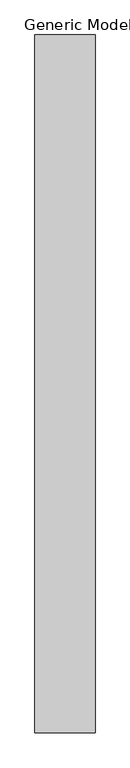
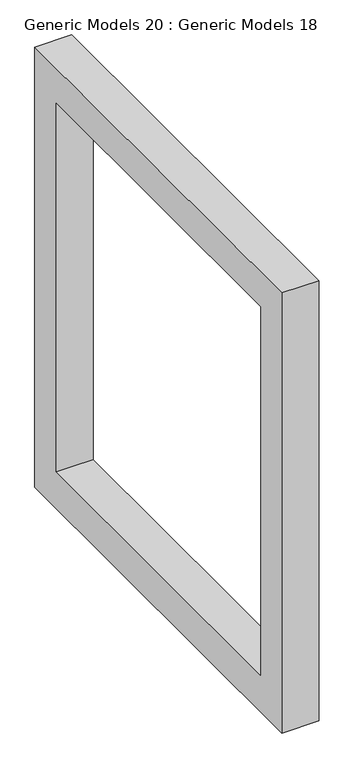
"""IFC4 building model written with IfcOpenShell, lengths in millimetres: proxy geometry, Generic Models 20 : Generic Models 18."""

from ifc_helpers import new_model, si_unit, frame, origin, place, context, project, spatial, polyline, outline, extrude, source, transform, mapped, element, save


def generic_models_20_generic_models_18_c69d9d0b(model_context):
    return source(origin(), model_context, "Body", "SweptSolid", [
        extrude(outline(polyline([(4881.9172538, 2692.4), (6355.1172538, 2692.4), (6355.1172538, 1092.2), (4881.9172538, 1092.2), (4881.9172538, 2692.4)]), holes=[polyline([(5008.9172538, 2565.4), (5008.9172538, 1225.55), (6228.1172538, 1225.55), (6228.1172538, 2565.4), (5008.9172538, 2565.4)])]), frame((-9825.1482439, 0.0, 0.0), z_axis=(1.0, 0.0, 0.0), x_axis=(0.0, 1.0, 0.0)), (0.0, 0.0, 1.0), 127.0),
    ])


if __name__ == "__main__":
    model = new_model("IFC4")
    model_context = context("Model", 3, world=origin())
    ifc_project = project(units=[si_unit("LENGTHUNIT", "METRE", prefix="MILLI")], contexts=[model_context])
    site = spatial("IfcSite", under=ifc_project)
    building = spatial("IfcBuilding", under=site)
    placement = place(None, origin())
    generic_models_20_generic_models_18_shape = generic_models_20_generic_models_18_c69d9d0b(model_context)
    element("IfcBuildingElementProxy", 1, Name="Generic Models 20 : Generic Models 18", ObjectType="Generic Models 20 : Generic Models 18", at=placement, inside=building, context=model_context, shape_type="MappedRepresentation", body=[
        mapped(generic_models_20_generic_models_18_shape, transform((0.0, 0.0, 0.0), x_axis=(1.0, 0.0, 0.0), y_axis=(0.0, 1.0, 0.0), z_axis=(0.0, 0.0, 1.0))),
    ])
    save(model, "model.ifc")

# Revit data of these elements
# Element 1 (IfcBuildingElementProxy, "Generic Models 20 : Generic Models 18")
#   Materials on its faces: "BLACK"
# Materials
#   "BLACK": class "Generic", colour RGB 120 120 120, transparency 0, Cost = 0
